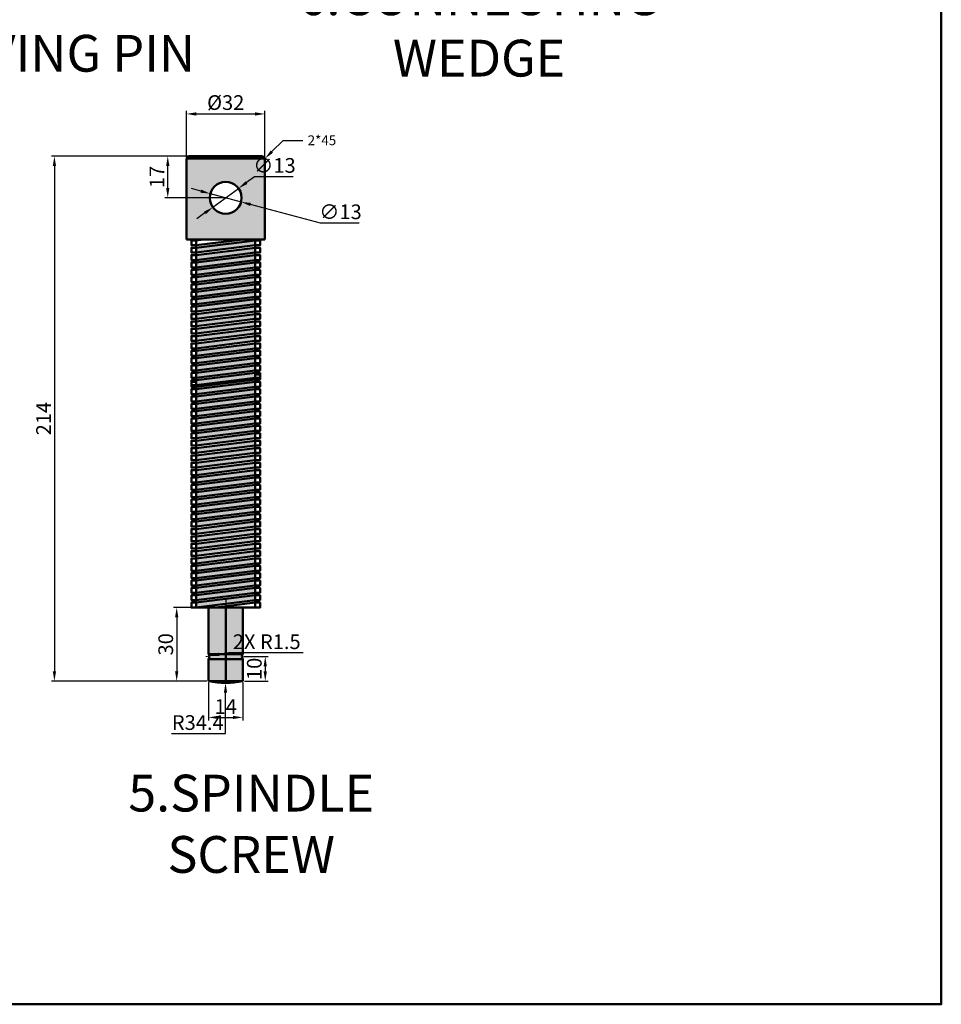
# Model space of a CAD drawing. Units: millimetres. Extents: x -14 to 1073, y -445 to 318.
# Tile 3 of 6: x 697 to 1073, y -445 to -44. Entities that reach past the tile are written whole.
import ezdxf
from ezdxf import colors
from ezdxf.entities.mleader import LeaderData, LeaderLine
from ezdxf.math import Vec2, Vec3

# ---------------------------------------------------------------- set-up
doc = ezdxf.new("R2010")
doc.units = ezdxf.units.MM
doc.header["$LTSCALE"] = 0.5
for name, color, linetype, lineweight in [('M-DIMS', 2, 'Continuous', 25), ('M-HATC', 8, 'Continuous', 18), ('M-OUTL', 7, 'Continuous', 50), ('M-TEXT', 3, 'Continuous', 25)]:
    doc.layers.add(name, color=color, linetype=linetype, lineweight=lineweight)
doc.styles.get("Standard").update_dxf_attribs({"font": 'arial.ttf'})
doc.dimstyles.new('ISO-25', dxfattribs={"dimtxt": 6, "dimasz": 4, "dimexe": 1.25, "dimexo": 0.625, "dimtad": 1, "dimtoh": 1, "dimtxsty": 'Standard', "dimcen": 2.5, "dimadec": 0, "dimazin": 0, "dimtfac": 1, "dimtmove": 0, "dimatfit": 3, "dimfxl": 1, "dimarcsym": 0})

# ---------------------------------------------------------------- blocks, each defined once
blk = doc.blocks.new('*D70')
at = {"layer": 'Defpoints', "color": 0, "ltscale": 0.5, "transparency": 16777216}
for p in [(797.07, -82.27), (765.07, -100.45), (797.07, -100.45)]:
    blk.add_point(p, dxfattribs=at)
at = {"layer": 'M-DIMS', "color": 0, "lineweight": -2, "ltscale": 0.5, "transparency": 16777216}
for p, q in [((765.07, -99.82), (765.07, -81.02)), ((769.07, -82.27), (793.07, -82.27)), ((797.07, -99.82), (797.07, -81.02))]:
    blk.add_line(p, q, dxfattribs=at)
at = {"layer": 'M-DIMS', "color": 0, "ltscale": 0.5, "transparency": 16777216}
for points in [[(769.07, -81.6), (769.07, -82.94), (765.07, -82.27)], [(793.07, -81.6), (793.07, -82.94), (797.07, -82.27)]]:
    blk.add_solid(points, dxfattribs=at)
at = {"layer": 'M-DIMS', "color": 0, "ltscale": 0.5, "transparency": 16777216, "insert": (781.07, -78.41), "char_height": 6, "attachment_point": 5}
blk.add_mtext('%%C32', dxfattribs=at)
blk = doc.blocks.new('*D71')
at = {"layer": 'Defpoints', "color": 0, "ltscale": 0.5, "transparency": 16777216}
for p in [(766.07, -99.45), (711.25, -313.45), (774.07, -313.45)]:
    blk.add_point(p, dxfattribs=at)
at = {"layer": 'M-DIMS', "color": 0, "lineweight": -2, "ltscale": 0.5, "transparency": 16777216}
for p, q in [((765.44, -99.45), (710, -99.45)), ((711.25, -103.45), (711.25, -309.45)), ((773.44, -313.45), (710, -313.45))]:
    blk.add_line(p, q, dxfattribs=at)
at = {"layer": 'M-DIMS', "color": 0, "ltscale": 0.5, "transparency": 16777216}
for points in [[(710.58, -103.45), (711.91, -103.45), (711.25, -99.45)], [(710.58, -309.45), (711.91, -309.45), (711.25, -313.45)]]:
    blk.add_solid(points, dxfattribs=at)
at = {"layer": 'M-DIMS', "color": 0, "ltscale": 0.5, "transparency": 16777216, "insert": (707.61, -206.45), "char_height": 6, "attachment_point": 5, "rotation": 90}
blk.add_mtext('214', dxfattribs=at)
blk = doc.blocks.new('*D72')
at = {"layer": 'Defpoints', "color": 0, "ltscale": 0.5, "transparency": 16777216}
for p in [(757.45, -99.45), (781.07, -99.45), (781.07, -116.45)]:
    blk.add_point(p, dxfattribs=at)
at = {"layer": 'M-DIMS', "color": 0, "lineweight": -2, "ltscale": 0.5, "transparency": 16777216}
for p, q in [((780.44, -99.45), (756.2, -99.45)), ((757.45, -112.45), (757.45, -103.45)), ((780.44, -116.45), (756.2, -116.45))]:
    blk.add_line(p, q, dxfattribs=at)
at = {"layer": 'M-DIMS', "color": 0, "ltscale": 0.5, "transparency": 16777216}
for points in [[(756.78, -103.45), (758.12, -103.45), (757.45, -99.45)], [(756.78, -112.45), (758.12, -112.45), (757.45, -116.45)]]:
    blk.add_solid(points, dxfattribs=at)
at = {"layer": 'M-DIMS', "color": 0, "ltscale": 0.5, "transparency": 16777216, "insert": (753.81, -107.95), "char_height": 6, "attachment_point": 5, "rotation": 90}
blk.add_mtext('17', dxfattribs=at)
blk = doc.blocks.new('*D73')
at = {"layer": 'Defpoints', "color": 0, "ltscale": 0.5, "transparency": 16777216}
for p in [(774.07, -313.45), (788.07, -313.45), (788.07, -328.24)]:
    blk.add_point(p, dxfattribs=at)
at = {"layer": 'M-DIMS', "color": 0, "lineweight": -2, "ltscale": 0.5, "transparency": 16777216}
for p, q in [((774.07, -314.07), (774.07, -329.49)), ((788.07, -314.07), (788.07, -329.49)), ((778.07, -328.24), (784.07, -328.24))]:
    blk.add_line(p, q, dxfattribs=at)
at = {"layer": 'M-DIMS', "color": 0, "ltscale": 0.5, "transparency": 16777216}
for points in [[(778.07, -327.57), (778.07, -328.9), (774.07, -328.24)], [(784.07, -327.57), (784.07, -328.9), (788.07, -328.24)]]:
    blk.add_solid(points, dxfattribs=at)
at = {"layer": 'M-DIMS', "color": 0, "ltscale": 0.5, "transparency": 16777216, "insert": (781.07, -324.6), "char_height": 6, "attachment_point": 5}
blk.add_mtext('14', dxfattribs=at)
blk = doc.blocks.new('*D74')
at = {"layer": 'Defpoints', "color": 0, "ltscale": 0.5, "transparency": 16777216}
for p in [(787.68, -303.45), (788.07, -313.45), (797.19, -313.45)]:
    blk.add_point(p, dxfattribs=at)
at = {"layer": 'M-DIMS', "color": 0, "lineweight": -2, "ltscale": 0.5, "transparency": 16777216}
for p, q in [((788.31, -303.45), (798.44, -303.45)), ((797.19, -307.45), (797.19, -309.45)), ((788.69, -313.45), (798.44, -313.45))]:
    blk.add_line(p, q, dxfattribs=at)
at = {"layer": 'M-DIMS', "color": 0, "ltscale": 0.5, "transparency": 16777216}
for points in [[(796.52, -307.45), (797.85, -307.45), (797.19, -303.45)], [(796.52, -309.45), (797.85, -309.45), (797.19, -313.45)]]:
    blk.add_solid(points, dxfattribs=at)
at = {"layer": 'M-DIMS', "color": 0, "ltscale": 0.5, "transparency": 16777216, "insert": (793.5, -308.45), "char_height": 6, "attachment_point": 5, "rotation": 90}
blk.add_mtext('10', dxfattribs=at)
blk = doc.blocks.new('*D75')
at = {"layer": 'Defpoints', "color": 0, "ltscale": 0.5, "transparency": 16777216}
for p in [(774.07, -283.45), (761.09, -313.45), (774.07, -313.45)]:
    blk.add_point(p, dxfattribs=at)
at = {"layer": 'M-DIMS', "color": 0, "lineweight": -2, "ltscale": 0.5, "transparency": 16777216}
for p, q in [((773.44, -283.45), (759.84, -283.45)), ((761.09, -287.45), (761.09, -309.45)), ((773.44, -313.45), (759.84, -313.45))]:
    blk.add_line(p, q, dxfattribs=at)
at = {"layer": 'M-DIMS', "color": 0, "ltscale": 0.5, "transparency": 16777216}
for points in [[(760.42, -287.45), (761.76, -287.45), (761.09, -283.45)], [(760.42, -309.45), (761.76, -309.45), (761.09, -313.45)]]:
    blk.add_solid(points, dxfattribs=at)
at = {"layer": 'M-DIMS', "color": 0, "ltscale": 0.5, "transparency": 16777216, "insert": (757.4, -298.45), "char_height": 6, "attachment_point": 5, "rotation": 90}
blk.add_mtext('30', dxfattribs=at)
blk = doc.blocks.new('*D76')
at = {"layer": 'Defpoints', "color": 0, "ltscale": 0.5, "transparency": 16777216}
for p in [(774.79, -114.76), (787.35, -118.13)]:
    blk.add_point(p, dxfattribs=at)
at = {"layer": 'M-DIMS', "color": 0, "lineweight": -2, "ltscale": 0.5, "transparency": 16777216}
for p, q in [((770.92, -113.73), (767.06, -112.7)), ((774.79, -114.76), (787.35, -118.13)), ((819.68, -126.78), (791.21, -119.16)), ((835.43, -126.78), (819.68, -126.78))]:
    blk.add_line(p, q, dxfattribs=at)
at = {"layer": 'M-DIMS', "color": 0, "ltscale": 0.5, "transparency": 16777216}
for points in [[(771.1, -113.09), (770.75, -114.37), (774.79, -114.76)], [(791.38, -118.52), (791.04, -119.8), (787.35, -118.13)]]:
    blk.add_solid(points, dxfattribs=at)
at = {"layer": 'M-DIMS', "color": 0, "ltscale": 0.5, "transparency": 16777216, "insert": (827.87, -122.93), "char_height": 6, "attachment_point": 5}
blk.add_mtext('∅13', dxfattribs=at)
blk = doc.blocks.new('*D88')
at = {"layer": 'Defpoints', "color": 0, "ltscale": 0.5, "transparency": 16777216}
for p in [(786.31, -112.61), (775.82, -120.28)]:
    blk.add_point(p, dxfattribs=at)
at = {"layer": 'M-DIMS', "color": 0, "lineweight": -2, "ltscale": 0.5, "transparency": 16777216}
for p, q in [((792.77, -107.89), (789.54, -110.25)), ((808.52, -107.89), (792.77, -107.89)), ((775.82, -120.28), (786.31, -112.61)), ((772.59, -122.64), (769.36, -125))]:
    blk.add_line(p, q, dxfattribs=at)
at = {"layer": 'M-DIMS', "color": 0, "ltscale": 0.5, "transparency": 16777216}
for points in [[(789.15, -109.71), (789.94, -110.79), (786.31, -112.61)], [(772.2, -122.1), (772.98, -123.18), (775.82, -120.28)]]:
    blk.add_solid(points, dxfattribs=at)
at = {"layer": 'M-DIMS', "color": 0, "ltscale": 0.5, "transparency": 16777216, "insert": (800.96, -104.03), "char_height": 6, "attachment_point": 5}
blk.add_mtext('∅13', dxfattribs=at)
blk = doc.blocks.new('*D89')
at = {"layer": 'Defpoints', "color": 0, "ltscale": 0.5, "transparency": 16777216}
for p in [(781.07, -279.76), (781, -314.16)]:
    blk.add_point(p, dxfattribs=at)
at = {"layer": 'M-DIMS', "color": 0, "lineweight": -2, "ltscale": 0.5, "transparency": 16777216}
for p, q in [((781.07, -279.76), (781, -314.16)), ((780.96, -334.81), (780.99, -318.16)), ((759.03, -334.81), (780.96, -334.81))]:
    blk.add_line(p, q, dxfattribs=at)
at = {"layer": 'M-DIMS', "color": 0, "ltscale": 0.5, "transparency": 16777216}
blk.add_solid([(780.33, -318.16), (781.66, -318.17), (781, -314.16)], dxfattribs=at)
at = {"layer": 'M-DIMS', "color": 0, "ltscale": 0.5, "transparency": 16777216, "insert": (769.68, -331.12), "char_height": 6, "attachment_point": 5}
blk.add_mtext('R34.4', dxfattribs=at)
blk = doc.blocks.new('*D90')
at = {"layer": 'Defpoints', "color": 0, "ltscale": 0.5, "transparency": 16777216}
for p in [(772.95, -303.45), (774.43, -303.2)]:
    blk.add_point(p, dxfattribs=at)
at = {"layer": 'M-DIMS', "color": 0, "lineweight": -2, "ltscale": 0.5, "transparency": 16777216}
for p, q in [((772.95, -303.45), (774.43, -303.2)), ((782.32, -301.86), (778.37, -302.53)), ((812.65, -301.86), (782.32, -301.86))]:
    blk.add_line(p, q, dxfattribs=at)
at = {"layer": 'M-DIMS', "color": 0, "ltscale": 0.5, "transparency": 16777216}
blk.add_solid([(778.26, -301.87), (778.48, -303.19), (774.43, -303.2)], dxfattribs=at)
at = {"layer": 'M-DIMS', "color": 0, "ltscale": 0.5, "transparency": 16777216, "insert": (797.79, -298.17), "char_height": 6, "attachment_point": 5}
blk.add_mtext('2X R1.5', dxfattribs=at)

msp = doc.modelspace()

# ---------------------------------------------------------------- hatches: boundary and pattern name
at = {"layer": 'M-HATC', "ltscale": 0.5}
h = msp.add_hatch(color=256, dxfattribs=at)
h.set_gradient(color1=(128, 128, 128), color2=(192, 192, 192), name='CYLINDER')
h.paths.add_polyline_path([(797.0663, -100.4452), (765.0663, -100.4452), (765.0663, -133.4452), (797.0663, -133.4452)])
h.paths.add_polyline_path([(774.5663, -116.4452, -1), (787.5663, -116.4452, -1)], flags=16)
h.paths.add_polyline_path([(796.0663, -99.4452), (766.0663, -99.4452), (765.0663, -100.4452), (797.0663, -100.4452)])
h.paths.add_polyline_path([(781.0663, -283.4452), (774.0663, -283.4452), (774.0663, -302.4452), (781.0663, -302.4452)])
h.paths.add_polyline_path([(788.0663, -283.4452), (781.0663, -283.4452), (781.0663, -302.4452), (788.0663, -302.4452)])
h.paths.add_polyline_path([(788.0663, -304.4452), (781.0663, -304.4452), (781.0663, -313.4452), (788.0663, -313.4452)])
h.paths.add_polyline_path([(788.0663, -302.4452), (781.0663, -302.4452), (781.0663, -304.4452), (788.0663, -304.4452, -0.38196601)])
h.paths.add_polyline_path([(781.0663, -302.4452), (774.0663, -302.4452, -0.38196601), (774.0663, -304.4452), (781.0663, -304.4452)])
h.paths.add_polyline_path([(781.0663, -304.4452), (774.0663, -304.4452), (774.0663, -313.4452), (781.0663, -313.4452)])
h.paths.add_polyline_path([(788.0663, -313.4452), (781.0663, -313.4452), (774.0663, -313.4452, 0.10281194)])
h.paths.add_polyline_path([(793.0663, -269.4452), (793.0663, -268.4452), (769.0663, -271.4452), (769.0663, -272.4452)])
h.paths.add_polyline_path([(793.0663, -271.4452), (793.0663, -269.4452), (769.0663, -272.4452), (769.0663, -274.4452)])
h.paths.add_polyline_path([(793.0663, -274.4452), (793.0663, -272.4452), (769.0663, -275.4452), (769.0663, -277.4452)])
h.paths.add_polyline_path([(793.0663, -277.4452), (793.0663, -275.4452), (769.0663, -278.4452), (769.0663, -280.4452)])
h.paths.add_polyline_path([(793.0663, -280.4452), (793.0663, -278.4452), (769.0663, -281.4452), (769.0663, -283.4452)])
h.paths.add_polyline_path([(793.0663, -268.4452), (793.0663, -266.4452), (769.0663, -269.4452), (769.0663, -271.4452)])
h.paths.add_polyline_path([(793.0663, -266.4452), (793.0663, -265.4452), (769.0663, -268.4452), (769.0663, -269.4452)])
h.paths.add_polyline_path([(793.0663, -263.4452), (769.0663, -266.4452), (769.0663, -268.4452), (793.0663, -265.4452)])
h.paths.add_polyline_path([(793.0663, -259.4452), (793.0663, -257.4452), (769.0663, -260.4452), (769.0663, -262.4452)])
h.paths.add_polyline_path([(793.0663, -256.4452), (793.0663, -254.4452), (769.0663, -257.4452), (769.0663, -259.4452)])
h.paths.add_polyline_path([(793.0663, -253.4452), (793.0663, -251.4452), (769.0663, -254.4452), (769.0663, -256.4452)])
h.paths.add_polyline_path([(793.0663, -247.4452), (793.0663, -245.4452), (769.0663, -248.4452), (769.0663, -250.4452)])
h.paths.add_polyline_path([(793.0663, -244.4452), (793.0663, -242.4452), (769.0663, -245.4452), (769.0663, -247.4452)])
h.paths.add_polyline_path([(793.0663, -241.4452), (793.0663, -239.4452), (769.0663, -242.4452), (769.0663, -244.4452)])
h.paths.add_polyline_path([(793.0663, -238.4452), (793.0663, -236.4452), (769.0663, -239.4452), (769.0663, -241.4452)])
h.paths.add_polyline_path([(793.0663, -235.4452), (793.0663, -233.4452), (769.0663, -236.4452), (769.0663, -238.4452)])
h.paths.add_polyline_path([(793.0663, -262.4452), (793.0663, -260.4452), (769.0663, -263.4452), (769.0663, -265.4452)])
h.paths.add_polyline_path([(793.0663, -250.4452), (793.0663, -248.4452), (769.0663, -251.4452), (769.0663, -253.4452)])
h.paths.add_polyline_path([(793.0663, -232.4452), (793.0663, -230.4452), (769.0663, -233.4452), (769.0663, -235.4452)])
h.paths.add_polyline_path([(793.0663, -229.4452), (793.0663, -227.4452), (769.0663, -230.4452), (769.0663, -232.4452)])
h.paths.add_polyline_path([(793.0663, -226.4452), (793.0663, -224.4452), (769.0663, -227.4452), (769.0663, -229.4452)])
h.paths.add_polyline_path([(793.0663, -223.4452), (793.0663, -221.4452), (769.0663, -224.4452), (769.0663, -226.4452)])
h.paths.add_polyline_path([(793.0663, -220.4452), (793.0663, -218.4452), (769.0663, -221.4452), (769.0663, -223.4452)])
h.paths.add_polyline_path([(793.0663, -217.4452), (793.0663, -215.4452), (769.0663, -218.4452), (769.0663, -220.4452)])
h.paths.add_polyline_path([(793.0663, -214.4452), (793.0663, -212.4452), (769.0663, -215.4452), (769.0663, -217.4452)])
h.paths.add_polyline_path([(793.0663, -211.4452), (793.0663, -209.4452), (769.0663, -212.4452), (769.0663, -214.4452)])
h.paths.add_polyline_path([(793.0663, -208.4452), (793.0663, -206.4452), (769.0663, -209.4452), (769.0663, -211.4452)])
h.paths.add_polyline_path([(793.0663, -205.4452), (793.0663, -203.4452), (769.0663, -206.4452), (769.0663, -208.4452)])
h.paths.add_polyline_path([(793.0663, -202.4452), (793.0663, -200.4452), (769.0663, -203.4452), (769.0663, -205.4452)])
h.paths.add_polyline_path([(793.0663, -193.4452), (793.0663, -191.4452), (769.0663, -194.4452), (769.0663, -196.4452)])
h.paths.add_polyline_path([(793.0663, -189.8112), (793.0663, -187.8112), (769.0663, -190.8112), (769.0663, -192.8112)])
h.paths.add_polyline_path([(793.0663, -169.8112), (769.0663, -172.8112), (769.0663, -174.8112), (793.0663, -171.8112)])
h.paths.add_polyline_path([(793.0663, -165.8112), (793.0663, -163.8112), (769.0663, -166.8112), (769.0663, -168.8112)])
h.paths.add_polyline_path([(793.0663, -138.8112), (769.0663, -141.8112), (769.0663, -142.8112), (793.0663, -139.8112)])
h.paths.add_polyline_path([(793.0663, -136.8112), (769.0663, -139.8112), (769.0663, -141.8112), (793.0663, -138.8112)])
h.paths.add_polyline_path([(793.0663, -133.8112), (793.0663, -133.4452), (787.9942, -133.4452), (769.0663, -135.8112), (769.0663, -136.8112)])
h.paths.add_polyline_path([(793.0663, -142.8112), (793.0663, -141.8112), (769.0663, -144.8112), (769.0663, -145.8112)])
h.paths.add_polyline_path([(793.0663, -154.8112), (793.0663, -153.8112), (769.0663, -156.8112), (769.0663, -157.8112)])
h.paths.add_polyline_path([(793.0663, -159.8112), (793.0663, -157.8112), (769.0663, -160.8112), (769.0663, -162.8112)])
h.paths.add_polyline_path([(793.0663, -168.8112), (793.0663, -166.8112), (769.0663, -169.8112), (769.0663, -171.8112)])
h.paths.add_polyline_path([(793.0663, -172.8112), (769.0663, -175.8112), (769.0663, -177.8112), (793.0663, -174.8112)])
h.paths.add_polyline_path([(793.0663, -181.8112), (769.0663, -184.8112), (769.0663, -186.8112), (793.0663, -183.8112)])
h.paths.add_polyline_path([(793.0663, -180.8112), (793.0663, -178.8112), (769.0663, -181.8112), (769.0663, -183.8112)])
h.paths.add_polyline_path([(793.0663, -153.8112), (793.0663, -151.8112), (769.0663, -154.8112), (769.0663, -156.8112)])
h.paths.add_polyline_path([(793.0663, -148.8112), (769.0663, -151.8112), (769.0663, -153.8112), (793.0663, -150.8112)])
h.paths.add_polyline_path([(793.0663, -147.8112), (793.0663, -145.8112), (769.0663, -148.8112), (769.0663, -150.8112)])
h.paths.add_polyline_path([(793.0663, -144.8112), (793.0663, -142.8112), (769.0663, -145.8112), (769.0663, -147.8112)])
h.paths.add_polyline_path([(793.0663, -157.8112), (793.0663, -156.8112), (769.0663, -159.8112), (769.0663, -160.8112)])
h.paths.add_polyline_path([(793.0663, -156.8112), (793.0663, -154.8112), (769.0663, -157.8112), (769.0663, -159.8112)])
h.paths.add_polyline_path([(793.0663, -162.8112), (793.0663, -160.8112), (769.0663, -163.8112), (769.0663, -165.8112)])
h.paths.add_polyline_path([(793.0663, -177.8112), (793.0663, -175.8112), (769.0663, -178.8112), (769.0663, -180.8112)])
h.paths.add_polyline_path([(793.0663, -186.8112), (793.0663, -184.8112), (769.0663, -187.8112), (769.0663, -189.8112)])
h.paths.add_polyline_path([(793.0663, -141.8112), (793.0663, -139.8112), (769.0663, -142.8112), (769.0663, -144.8112)])
h.paths.add_polyline_path([(793.0663, -196.4452), (793.0663, -194.4452), (769.0663, -197.4452), (769.0663, -199.4452)])
h.paths.add_polyline_path([(793.0663, -200.4452), (793.0663, -199.4452), (769.0663, -202.4452), (769.0663, -203.4452)])
h.paths.add_polyline_path([(793.0663, -199.4452), (793.0663, -197.4452), (769.0663, -200.4452), (769.0663, -202.4452)])
h.paths.add_polyline_path([(793.0663, -135.8112), (793.0663, -133.8112), (769.0663, -136.8112), (769.0663, -138.8112)])
h.paths.add_polyline_path([(793.0663, -190.4452), (793.0663, -189.8112), (769.0663, -192.8112), (769.0663, -193.4452)])
h.paths.add_polyline_path([(793.0663, -191.4452), (793.0663, -190.4452), (769.0663, -193.4452), (769.0663, -194.4452)])

# ---------------------------------------------------------------- linework, layer by layer
at = {"layer": 'M-OUTL', "ltscale": 0.5}
for p, q in [((766.0663, -99.4452), (765.0663, -100.4452)), ((766.0663, -99.4452), (796.0663, -99.4452)), ((796.0663, -99.4452), (797.0663, -100.4452)), ((765.0663, -133.4452), (765.0663, -100.4452)), ((765.0663, -100.4452), (797.0663, -100.4452)), ((797.0663, -100.4452), (797.0663, -133.4452)), ((797.0663, -133.4452), (765.0663, -133.4452)), ((769.0663, -133.4452), (769.0663, -283.4452)), ((769.0663, -133.8112), (771.9942, -133.4452)), ((769.0663, -135.8112), (787.9942, -133.4452)), ((769.0663, -136.8112), (793.0663, -133.8112)), ((769.0663, -138.8112), (793.0663, -135.8112)), ((793.0663, -133.4452), (793.0663, -283.4452)), ((769.0663, -139.8112), (793.0663, -136.8112)), ((769.0663, -141.8112), (793.0663, -138.8112)), ((769.0663, -142.8112), (793.0663, -139.8112)), ((769.0663, -144.8112), (793.0663, -141.8112)), ((769.0663, -145.8112), (793.0663, -142.8112)), ((769.0663, -147.8112), (793.0663, -144.8112)), ((769.0663, -148.8112), (793.0663, -145.8112)), ((769.0663, -150.8112), (793.0663, -147.8112)), ((769.0663, -151.8112), (793.0663, -148.8112)), ((769.0663, -153.8112), (793.0663, -150.8112)), ((769.0663, -154.8112), (793.0663, -151.8112)), ((769.0663, -156.8112), (793.0663, -153.8112)), ((769.0663, -157.8112), (793.0663, -154.8112)), ((769.0663, -159.8112), (793.0663, -156.8112)), ((769.0663, -160.8112), (793.0663, -157.8112)), ((769.0663, -162.8112), (793.0663, -159.8112)), ((769.0663, -163.8112), (793.0663, -160.8112)), ((769.0663, -165.8112), (793.0663, -162.8112)), ((769.0663, -166.8112), (793.0663, -163.8112)), ((769.0663, -168.8112), (793.0663, -165.8112)), ((769.0663, -169.8112), (793.0663, -166.8112)), ((769.0663, -171.8112), (793.0663, -168.8112)), ((769.0663, -172.8112), (793.0663, -169.8112)), ((769.0663, -174.8112), (793.0663, -171.8112)), ((769.0663, -175.8112), (793.0663, -172.8112)), ((769.0663, -177.8112), (793.0663, -174.8112)), ((769.0663, -178.8112), (793.0663, -175.8112)), ((769.0663, -180.8112), (793.0663, -177.8112)), ((769.0663, -181.8112), (793.0663, -178.8112)), ((769.0663, -183.8112), (793.0663, -180.8112)), ((769.0663, -184.8112), (793.0663, -181.8112)), ((769.0663, -186.8112), (793.0663, -183.8112)), ((769.0663, -187.8112), (793.0663, -184.8112)), ((769.0663, -189.8112), (793.0663, -186.8112)), ((769.0663, -190.8112), (793.0663, -187.8112)), ((769.0663, -192.8112), (793.0663, -189.8112)), ((769.0663, -193.4452), (793.0663, -190.4452)), ((769.0663, -194.4452), (793.0663, -191.4452)), ((769.0663, -196.4452), (793.0663, -193.4452)), ((769.0663, -197.4452), (793.0663, -194.4452)), ((769.0663, -199.4452), (793.0663, -196.4452)), ((769.0663, -200.4452), (793.0663, -197.4452)), ((769.0663, -202.4452), (793.0663, -199.4452)), ((769.0663, -203.4452), (793.0663, -200.4452)), ((769.0663, -205.4452), (793.0663, -202.4452)), ((769.0663, -206.4452), (793.0663, -203.4452)), ((769.0663, -208.4452), (793.0663, -205.4452)), ((769.0663, -209.4452), (793.0663, -206.4452)), ((769.0663, -211.4452), (793.0663, -208.4452)), ((769.0663, -212.4452), (793.0663, -209.4452)), ((769.0663, -214.4452), (793.0663, -211.4452)), ((769.0663, -215.4452), (793.0663, -212.4452)), ((769.0663, -217.4452), (793.0663, -214.4452)), ((769.0663, -218.4452), (793.0663, -215.4452)), ((769.0663, -220.4452), (793.0663, -217.4452)), ((769.0663, -221.4452), (793.0663, -218.4452)), ((769.0663, -223.4452), (793.0663, -220.4452)), ((769.0663, -224.4452), (793.0663, -221.4452)), ((769.0663, -226.4452), (793.0663, -223.4452)), ((769.0663, -227.4452), (793.0663, -224.4452)), ((769.0663, -229.4452), (793.0663, -226.4452)), ((769.0663, -230.4452), (793.0663, -227.4452)), ((769.0663, -232.4452), (793.0663, -229.4452)), ((769.0663, -233.4452), (793.0663, -230.4452)), ((769.0663, -235.4452), (793.0663, -232.4452)), ((769.0663, -236.4452), (793.0663, -233.4452)), ((769.0663, -236.4452), (793.0663, -233.4452)), ((769.0663, -238.4452), (793.0663, -235.4452)), ((769.0663, -238.4452), (793.0663, -235.4452)), ((769.0663, -239.4452), (793.0663, -236.4452)), ((769.0663, -239.4452), (793.0663, -236.4452)), ((769.0663, -241.4452), (793.0663, -238.4452)), ((769.0663, -241.4452), (793.0663, -238.4452)), ((769.0663, -242.4452), (793.0663, -239.4452)), ((769.0663, -244.4452), (793.0663, -241.4452)), ((769.0663, -245.4452), (793.0663, -242.4452)), ((769.0663, -247.4452), (793.0663, -244.4452)), ((769.0663, -248.4452), (793.0663, -245.4452)), ((769.0663, -250.4452), (793.0663, -247.4452)), ((769.0663, -251.4452), (793.0663, -248.4452)), ((769.0663, -253.4452), (793.0663, -250.4452)), ((769.0663, -254.4452), (793.0663, -251.4452)), ((769.0663, -256.4452), (793.0663, -253.4452)), ((769.0663, -257.4452), (793.0663, -254.4452)), ((769.0663, -259.4452), (793.0663, -256.4452)), ((769.0663, -260.4452), (793.0663, -257.4452)), ((769.0663, -262.4452), (793.0663, -259.4452)), ((769.0663, -263.4452), (793.0663, -260.4452)), ((769.0663, -265.4452), (793.0663, -262.4452)), ((769.0663, -266.4452), (793.0663, -263.4452)), ((769.0663, -268.4452), (793.0663, -265.4452)), ((769.0663, -269.4452), (793.0663, -266.4452)), ((769.0663, -271.4452), (793.0663, -268.4452)), ((769.0663, -272.4452), (793.0663, -269.4452)), ((769.0663, -274.4452), (793.0663, -271.4452)), ((769.0663, -275.4452), (793.0663, -272.4452)), ((769.0663, -277.4452), (793.0663, -274.4452)), ((769.0663, -278.4452), (793.0663, -275.4452)), ((769.0663, -280.4452), (793.0663, -277.4452)), ((769.0663, -281.4452), (793.0663, -278.4452)), ((769.0663, -283.4452), (793.0663, -280.4452)), ((769.0663, -283.4452), (793.0663, -283.4452)), ((774.0663, -283.4452), (774.0663, -302.4452)), ((777.0663, -283.4452), (793.0663, -281.4452)), ((781.0663, -283.4452), (781.0663, -313.4452)), ((788.0663, -283.4452), (788.0663, -302.4452)), ((774.0663, -302.4452), (788.0663, -302.4452)), ((774.0663, -304.4452), (788.0663, -304.4452)), ((774.0663, -304.4452), (774.0663, -313.4452)), ((788.0663, -304.4452), (788.0663, -313.4452)), ((774.0663, -313.4452), (788.0663, -313.4452))]:
    msp.add_line(p, q, dxfattribs=at)
msp.add_lwpolyline([(-13.7695, 318.0907), (1072.7514, 318.0907), (1072.7514, -445.1795), (-13.7695, -445.1795)], close=True, dxfattribs=at)
for points in [[(769.0663, -133.8112), (767.0663, -133.8112), (767.0663, -135.8112), (769.0663, -135.8112)], [(793.0663, -133.8112), (795.0663, -133.8112), (795.0663, -135.8112), (793.0663, -135.8112)], [(769.0663, -136.8112), (767.0663, -136.8112), (767.0663, -138.8112), (769.0663, -138.8112)], [(769.0663, -139.8112), (767.0663, -139.8112), (767.0663, -141.8112), (769.0663, -141.8112)], [(793.0663, -136.8112), (795.0663, -136.8112), (795.0663, -138.8112), (793.0663, -138.8112)], [(793.0663, -139.8112), (795.0663, -139.8112), (795.0663, -141.8112), (793.0663, -141.8112)], [(769.0663, -142.8112), (767.0663, -142.8112), (767.0663, -144.8112), (769.0663, -144.8112)], [(793.0663, -142.8112), (795.0663, -142.8112), (795.0663, -144.8112), (793.0663, -144.8112)], [(769.0663, -145.8112), (767.0663, -145.8112), (767.0663, -147.8112), (769.0663, -147.8112)], [(793.0663, -145.8112), (795.0663, -145.8112), (795.0663, -147.8112), (793.0663, -147.8112)], [(769.0663, -148.8112), (767.0663, -148.8112), (767.0663, -150.8112), (769.0663, -150.8112)], [(769.0663, -151.8112), (767.0663, -151.8112), (767.0663, -153.8112), (769.0663, -153.8112)], [(793.0663, -148.8112), (795.0663, -148.8112), (795.0663, -150.8112), (793.0663, -150.8112)], [(793.0663, -151.8112), (795.0663, -151.8112), (795.0663, -153.8112), (793.0663, -153.8112)], [(769.0663, -154.8112), (767.0663, -154.8112), (767.0663, -156.8112), (769.0663, -156.8112)], [(793.0663, -154.8112), (795.0663, -154.8112), (795.0663, -156.8112), (793.0663, -156.8112)], [(769.0663, -157.8112), (767.0663, -157.8112), (767.0663, -159.8112), (769.0663, -159.8112)], [(793.0663, -157.8112), (795.0663, -157.8112), (795.0663, -159.8112), (793.0663, -159.8112)], [(769.0663, -160.8112), (767.0663, -160.8112), (767.0663, -162.8112), (769.0663, -162.8112)], [(769.0663, -163.8112), (767.0663, -163.8112), (767.0663, -165.8112), (769.0663, -165.8112)], [(793.0663, -160.8112), (795.0663, -160.8112), (795.0663, -162.8112), (793.0663, -162.8112)], [(793.0663, -163.8112), (795.0663, -163.8112), (795.0663, -165.8112), (793.0663, -165.8112)], [(769.0663, -166.8112), (767.0663, -166.8112), (767.0663, -168.8112), (769.0663, -168.8112)], [(793.0663, -166.8112), (795.0663, -166.8112), (795.0663, -168.8112), (793.0663, -168.8112)], [(769.0663, -169.8112), (767.0663, -169.8112), (767.0663, -171.8112), (769.0663, -171.8112)], [(793.0663, -169.8112), (795.0663, -169.8112), (795.0663, -171.8112), (793.0663, -171.8112)], [(769.0663, -172.8112), (767.0663, -172.8112), (767.0663, -174.8112), (769.0663, -174.8112)], [(769.0663, -175.8112), (767.0663, -175.8112), (767.0663, -177.8112), (769.0663, -177.8112)], [(793.0663, -172.8112), (795.0663, -172.8112), (795.0663, -174.8112), (793.0663, -174.8112)], [(793.0663, -175.8112), (795.0663, -175.8112), (795.0663, -177.8112), (793.0663, -177.8112)], [(769.0663, -178.8112), (767.0663, -178.8112), (767.0663, -180.8112), (769.0663, -180.8112)], [(793.0663, -178.8112), (795.0663, -178.8112), (795.0663, -180.8112), (793.0663, -180.8112)], [(769.0663, -181.8112), (767.0663, -181.8112), (767.0663, -183.8112), (769.0663, -183.8112)], [(793.0663, -181.8112), (795.0663, -181.8112), (795.0663, -183.8112), (793.0663, -183.8112)], [(769.0663, -184.8112), (767.0663, -184.8112), (767.0663, -186.8112), (769.0663, -186.8112)], [(769.0663, -187.8112), (767.0663, -187.8112), (767.0663, -189.8112), (769.0663, -189.8112)], [(793.0663, -184.8112), (795.0663, -184.8112), (795.0663, -186.8112), (793.0663, -186.8112)], [(793.0663, -187.8112), (795.0663, -187.8112), (795.0663, -189.8112), (793.0663, -189.8112)], [(793.0663, -188.4452), (795.0663, -188.4452), (795.0663, -190.4452), (793.0663, -190.4452)], [(769.0663, -190.8112), (767.0663, -190.8112), (767.0663, -192.8112), (769.0663, -192.8112)], [(769.0663, -191.4452), (767.0663, -191.4452), (767.0663, -193.4452), (769.0663, -193.4452)], [(793.0663, -191.4452), (795.0663, -191.4452), (795.0663, -193.4452), (793.0663, -193.4452)], [(769.0663, -194.4452), (767.0663, -194.4452), (767.0663, -196.4452), (769.0663, -196.4452)], [(793.0663, -194.4452), (795.0663, -194.4452), (795.0663, -196.4452), (793.0663, -196.4452)], [(769.0663, -197.4452), (767.0663, -197.4452), (767.0663, -199.4452), (769.0663, -199.4452)], [(769.0663, -200.4452), (767.0663, -200.4452), (767.0663, -202.4452), (769.0663, -202.4452)], [(793.0663, -197.4452), (795.0663, -197.4452), (795.0663, -199.4452), (793.0663, -199.4452)], [(793.0663, -200.4452), (795.0663, -200.4452), (795.0663, -202.4452), (793.0663, -202.4452)], [(769.0663, -203.4452), (767.0663, -203.4452), (767.0663, -205.4452), (769.0663, -205.4452)], [(793.0663, -203.4452), (795.0663, -203.4452), (795.0663, -205.4452), (793.0663, -205.4452)], [(769.0663, -206.4452), (767.0663, -206.4452), (767.0663, -208.4452), (769.0663, -208.4452)], [(793.0663, -206.4452), (795.0663, -206.4452), (795.0663, -208.4452), (793.0663, -208.4452)], [(769.0663, -209.4452), (767.0663, -209.4452), (767.0663, -211.4452), (769.0663, -211.4452)], [(769.0663, -212.4452), (767.0663, -212.4452), (767.0663, -214.4452), (769.0663, -214.4452)], [(793.0663, -209.4452), (795.0663, -209.4452), (795.0663, -211.4452), (793.0663, -211.4452)], [(793.0663, -212.4452), (795.0663, -212.4452), (795.0663, -214.4452), (793.0663, -214.4452)], [(769.0663, -215.4452), (767.0663, -215.4452), (767.0663, -217.4452), (769.0663, -217.4452)], [(793.0663, -215.4452), (795.0663, -215.4452), (795.0663, -217.4452), (793.0663, -217.4452)], [(769.0663, -218.4452), (767.0663, -218.4452), (767.0663, -220.4452), (769.0663, -220.4452)], [(793.0663, -218.4452), (795.0663, -218.4452), (795.0663, -220.4452), (793.0663, -220.4452)], [(769.0663, -221.4452), (767.0663, -221.4452), (767.0663, -223.4452), (769.0663, -223.4452)], [(769.0663, -224.4452), (767.0663, -224.4452), (767.0663, -226.4452), (769.0663, -226.4452)], [(793.0663, -221.4452), (795.0663, -221.4452), (795.0663, -223.4452), (793.0663, -223.4452)], [(793.0663, -224.4452), (795.0663, -224.4452), (795.0663, -226.4452), (793.0663, -226.4452)], [(769.0663, -227.4452), (767.0663, -227.4452), (767.0663, -229.4452), (769.0663, -229.4452)], [(793.0663, -227.4452), (795.0663, -227.4452), (795.0663, -229.4452), (793.0663, -229.4452)], [(769.0663, -230.4452), (767.0663, -230.4452), (767.0663, -232.4452), (769.0663, -232.4452)], [(793.0663, -230.4452), (795.0663, -230.4452), (795.0663, -232.4452), (793.0663, -232.4452)], [(769.0663, -233.4452), (767.0663, -233.4452), (767.0663, -235.4452), (769.0663, -235.4452)], [(769.0663, -236.4452), (767.0663, -236.4452), (767.0663, -238.4452), (769.0663, -238.4452)], [(769.0663, -236.4452), (767.0663, -236.4452), (767.0663, -238.4452), (769.0663, -238.4452)], [(793.0663, -233.4452), (795.0663, -233.4452), (795.0663, -235.4452), (793.0663, -235.4452)], [(793.0663, -233.4452), (795.0663, -233.4452), (795.0663, -235.4452), (793.0663, -235.4452)], [(793.0663, -236.4452), (795.0663, -236.4452), (795.0663, -238.4452), (793.0663, -238.4452)], [(793.0663, -236.4452), (795.0663, -236.4452), (795.0663, -238.4452), (793.0663, -238.4452)], [(769.0663, -239.4452), (767.0663, -239.4452), (767.0663, -241.4452), (769.0663, -241.4452)], [(769.0663, -239.4452), (767.0663, -239.4452), (767.0663, -241.4452), (769.0663, -241.4452)], [(793.0663, -239.4452), (795.0663, -239.4452), (795.0663, -241.4452), (793.0663, -241.4452)], [(769.0663, -242.4452), (767.0663, -242.4452), (767.0663, -244.4452), (769.0663, -244.4452)], [(793.0663, -242.4452), (795.0663, -242.4452), (795.0663, -244.4452), (793.0663, -244.4452)], [(769.0663, -245.4452), (767.0663, -245.4452), (767.0663, -247.4452), (769.0663, -247.4452)], [(769.0663, -248.4452), (767.0663, -248.4452), (767.0663, -250.4452), (769.0663, -250.4452)], [(793.0663, -245.4452), (795.0663, -245.4452), (795.0663, -247.4452), (793.0663, -247.4452)], [(793.0663, -248.4452), (795.0663, -248.4452), (795.0663, -250.4452), (793.0663, -250.4452)], [(769.0663, -251.4452), (767.0663, -251.4452), (767.0663, -253.4452), (769.0663, -253.4452)], [(793.0663, -251.4452), (795.0663, -251.4452), (795.0663, -253.4452), (793.0663, -253.4452)], [(769.0663, -254.4452), (767.0663, -254.4452), (767.0663, -256.4452), (769.0663, -256.4452)], [(793.0663, -254.4452), (795.0663, -254.4452), (795.0663, -256.4452), (793.0663, -256.4452)], [(769.0663, -257.4452), (767.0663, -257.4452), (767.0663, -259.4452), (769.0663, -259.4452)], [(769.0663, -260.4452), (767.0663, -260.4452), (767.0663, -262.4452), (769.0663, -262.4452)], [(793.0663, -257.4452), (795.0663, -257.4452), (795.0663, -259.4452), (793.0663, -259.4452)], [(793.0663, -260.4452), (795.0663, -260.4452), (795.0663, -262.4452), (793.0663, -262.4452)], [(769.0663, -263.4452), (767.0663, -263.4452), (767.0663, -265.4452), (769.0663, -265.4452)], [(793.0663, -263.4452), (795.0663, -263.4452), (795.0663, -265.4452), (793.0663, -265.4452)], [(769.0663, -266.4452), (767.0663, -266.4452), (767.0663, -268.4452), (769.0663, -268.4452)], [(793.0663, -266.4452), (795.0663, -266.4452), (795.0663, -268.4452), (793.0663, -268.4452)], [(769.0663, -269.4452), (767.0663, -269.4452), (767.0663, -271.4452), (769.0663, -271.4452)], [(769.0663, -272.4452), (767.0663, -272.4452), (767.0663, -274.4452), (769.0663, -274.4452)], [(793.0663, -269.4452), (795.0663, -269.4452), (795.0663, -271.4452), (793.0663, -271.4452)], [(793.0663, -272.4452), (795.0663, -272.4452), (795.0663, -274.4452), (793.0663, -274.4452)], [(769.0663, -275.4452), (767.0663, -275.4452), (767.0663, -277.4452), (769.0663, -277.4452)], [(793.0663, -275.4452), (795.0663, -275.4452), (795.0663, -277.4452), (793.0663, -277.4452)], [(769.0663, -278.4452), (767.0663, -278.4452), (767.0663, -280.4452), (769.0663, -280.4452)], [(793.0663, -278.4452), (795.0663, -278.4452), (795.0663, -280.4452), (793.0663, -280.4452)], [(769.0663, -281.4452), (767.0663, -281.4452), (767.0663, -283.4452), (769.0663, -283.4452)], [(793.0663, -281.4452), (795.0663, -281.4452), (795.0663, -283.4452), (793.0663, -283.4452)]]:
    msp.add_lwpolyline(points, dxfattribs=at)
msp.add_circle((781.0663, -116.4452), 6.5, dxfattribs=at)
for centre, radius, start, end in [((772.9483, -303.4452), 1.5, 318.189685, 41.810315), ((789.1843, -303.4452), 1.5, 138.189685, 221.810315), ((781.0663, -279.7623), 34.4026, 258.259869, 281.740131)]:
    msp.add_arc(centre, radius, start, end, dxfattribs=at)

# ---------------------------------------------------------------- texts
at = {"layer": 'M-TEXT', "ltscale": 0.5, "char_height": 15, "attachment_point": 1}
for s, width, insert in [('\\pxqc;6.CONNECTING WEDGE', 218.927832, (774.8768, -27.0126)), ('\\pxqc;10.MOVING PIN', 154.431653, (618.8169, -50.0413)), ('\\pxqc;5.SPINDLE SCREW', 154.431653, (714.2576, -351.5985))]:
    msp.add_mtext_dynamic_manual_height_columns(s, width=width, gutter_width=12.5, heights=[0], dxfattribs=dict(at, insert=insert))

# ---------------------------------------------------------------- dimensions: what is measured, and where the dimension line sits
at = {"layer": 'M-DIMS', "ltscale": 0.5}
dim = msp.add_linear_dim(base=(797.0663, -82.2705), p1=(765.0663, -100.4452), p2=(797.0663, -100.4452), text='%%C<>', dimstyle='ISO-25', override={"dimclrd": 0, "dimclre": 0, "dimclrt": 0}, dxfattribs=at)
dim.commit()
dim.dimension.update_dxf_attribs({"geometry": '*D70', "text_midpoint": (781.0663, -78.4142)})
for base, p1, p2, picture, middle in [((711.2477, -313.4452), (766.0663, -99.4452), (774.0663, -313.4452), '*D71', (707.6105, -206.4452)), ((757.4508, -99.4452), (781.0663, -116.4452), (781.0663, -99.4452), '*D72', (753.8136, -107.9452)), ((761.0897, -313.4452), (774.0663, -283.4452), (774.0663, -313.4452), '*D75', (757.3992, -298.4452)), ((797.1859, -313.4452), (787.6843, -303.4452), (788.0663, -313.4452), '*D74', (793.4975, -308.4452))]:
    dim = msp.add_linear_dim(base=base, p1=p1, p2=p2, angle=90, dimstyle='ISO-25', override={"dimclrd": 0, "dimclre": 0, "dimclrt": 0}, dxfattribs=at)
    dim.commit()
    dim.dimension.update_dxf_attribs({"geometry": picture, "text_midpoint": middle})
for p1, p2, override, picture, middle in [((775.8188, -120.2811), (786.3137, -112.6093), {"dimdec": 0, "dimlfac": 1, "dimrnd": 0, "dimzin": 0, "dimdsep": 46, "dimlunit": 2}, '*D88', (800.9585, -107.8881)), ((774.7873, -114.7646), (787.3453, -118.1258), {"dimclrd": 0, "dimclre": 0, "dimclrt": 0}, '*D76', (819.6849, -126.7814))]:
    dim = msp.add_diameter_dim_2p(p1=p1, p2=p2, dimstyle='ISO-25', override=override, dxfattribs=at)
    dim.commit()
    dim.dimension.update_dxf_attribs({"geometry": picture, "text_midpoint": middle, "dimtype": 163})
dim = msp.add_radius_dim(center=(781.0663, -279.7623), mpoint=(781.0001, -314.1648), dimstyle='ISO-25', override={"dimdec": 1, "dimlfac": 1, "dimrnd": 0, "dimzin": 0, "dimdsep": 46, "dimlunit": 2}, dxfattribs=at)
dim.commit()
dim.dimension.update_dxf_attribs({"geometry": '*D89', "text_midpoint": (769.6839, -334.8063), "dimtype": 164})
dim = msp.add_radius_dim(center=(772.9483, -303.4452), mpoint=(774.4273, -303.1954), text='2X <>', dimstyle='ISO-25', override={"dimdec": 1, "dimlfac": 1, "dimrnd": 0, "dimzin": 0, "dimdsep": 46, "dimlunit": 2}, dxfattribs=at)
dim.commit()
dim.dimension.update_dxf_attribs({"geometry": '*D90', "text_midpoint": (797.7932, -298.1746)})
dim = msp.add_linear_dim(base=(788.0663, -328.2353), p1=(774.0663, -313.4452), p2=(788.0663, -313.4452), dimstyle='ISO-25', override={"dimclrd": 0, "dimclre": 0, "dimclrt": 0}, dxfattribs=at)
dim.commit()
dim.dimension.update_dxf_attribs({"geometry": '*D73', "text_midpoint": (781.0663, -324.598)})

# ---------------------------------------------------------------- leaders
ml = msp.add_multileader_mtext('Standard', dxfattribs=at)
ml.set_content('2*45', color=256)
ml.set_leader_properties()
ml.build(insert=Vec2(0, 0))
ctx = ml.context
ctx.base_point, ctx.plane_origin = Vec3(812.4734, -93.0381), Vec3(797.0663, -100.4452)
notes = []
notes.append((ctx, [(0, (1, 1, 0), (804.4734, -93.0381), (1, 0), 8, [(0, [(797.0663, -100.4452)], 0, [])])]))
ctx.mtext.insert, ctx.mtext.flow_direction = Vec3(814.4734, -91.004), 5
for ctx, leaders in notes:
    for number, flags, end, landing, length, lines in leaders:
        leader = LeaderData()
        leader.index, (leader.has_last_leader_line, leader.has_dogleg_vector, leader.attachment_direction) = number, flags
        leader.last_leader_point, leader.dogleg_vector, leader.dogleg_length = Vec3(end), Vec3(landing), length
        for number, points, colour, breaks in lines:
            line = LeaderLine()
            line.index, line.vertices, line.color, line.breaks = number, Vec3.list(points), colors.encode_raw_color(colour), breaks
            leader.lines.append(line)
        ctx.leaders.append(leader)

doc.saveas('drawing.dxf')
